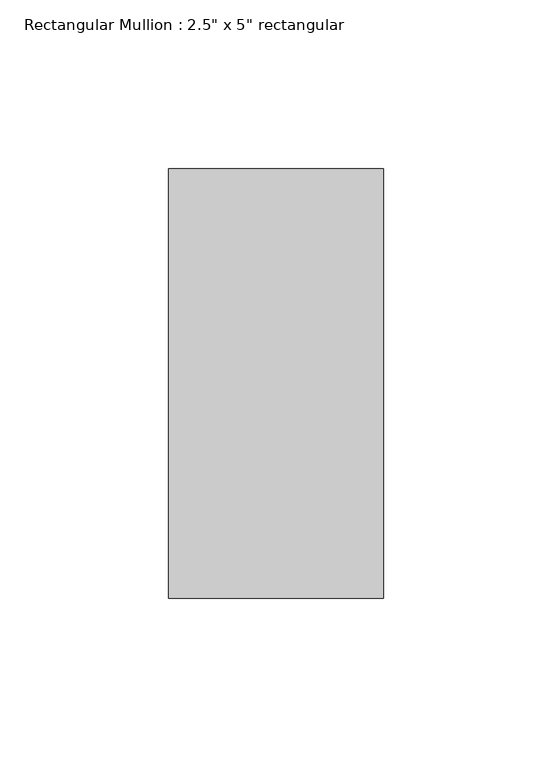
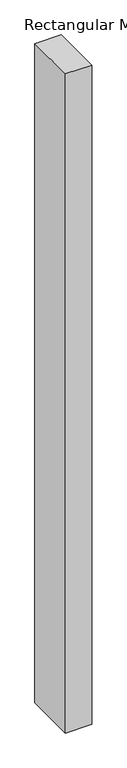
"""IFC4 building model written with IfcOpenShell, lengths in millimetres: member geometry."""

from ifc_helpers import new_model, si_unit, frame, origin, place, context, project, spatial, polyline, outline, extrude, source, transform, mapped, element, save


def member_0c6ed757(model_context):
    return source(origin(), model_context, "Body", "SweptSolid", [
        extrude(outline(polyline([(31.75, 63.5), (31.75, -63.5), (-31.75, -63.5), (-31.75, 63.5), (31.75, 63.5)])), frame((0.0, 0.0, -1678.8095798), z_axis=(0.0, 0.0, 1.0), x_axis=(1.0, 0.0, 0.0)), (0.0, 0.0, 1.0), 1678.8095798),
    ])


if __name__ == "__main__":
    model = new_model("IFC4")
    model_context = context("Model", 3, world=origin())
    ifc_project = project(units=[si_unit("LENGTHUNIT", "METRE", prefix="MILLI")], contexts=[model_context])
    site = spatial("IfcSite", under=ifc_project)
    building = spatial("IfcBuilding", under=site)
    placement = place(None, origin())
    member_shape = member_0c6ed757(model_context)
    element("IfcMember", 1, ObjectType="Rectangular Mullion : 2.5\" x 5\" rectangular", at=placement, inside=building, context=model_context, shape_type="MappedRepresentation", body=[
        mapped(member_shape, transform((0.0, 0.0, 0.0), x_axis=(1.0, 0.0, 0.0), y_axis=(0.0, 1.0, 0.0), z_axis=(0.0, 0.0, 1.0))),
    ])
    save(model, "model.ifc")

# Revit data of these elements
# Type "Rectangular Mullion : 2.5\" x 5\" rectangular"
#   built-in parameter 1007304 = 0.416667 (stored number, unit not read)
#   built-in parameter 1007301 = 0.104167 (stored number, unit not read)
#   built-in parameter 1007300 = 0.104167 (stored number, unit not read)
# Element 1 (IfcMember, "Rectangular Mullion : 2.5\" x 5\" rectangular")
#   Materials on its faces: "Aluminum"
# Materials
#   "Aluminum": class "Metal", colour RGB 247 247 247, transparency 0, Description = "Aluminum 6061", Cost = 0
